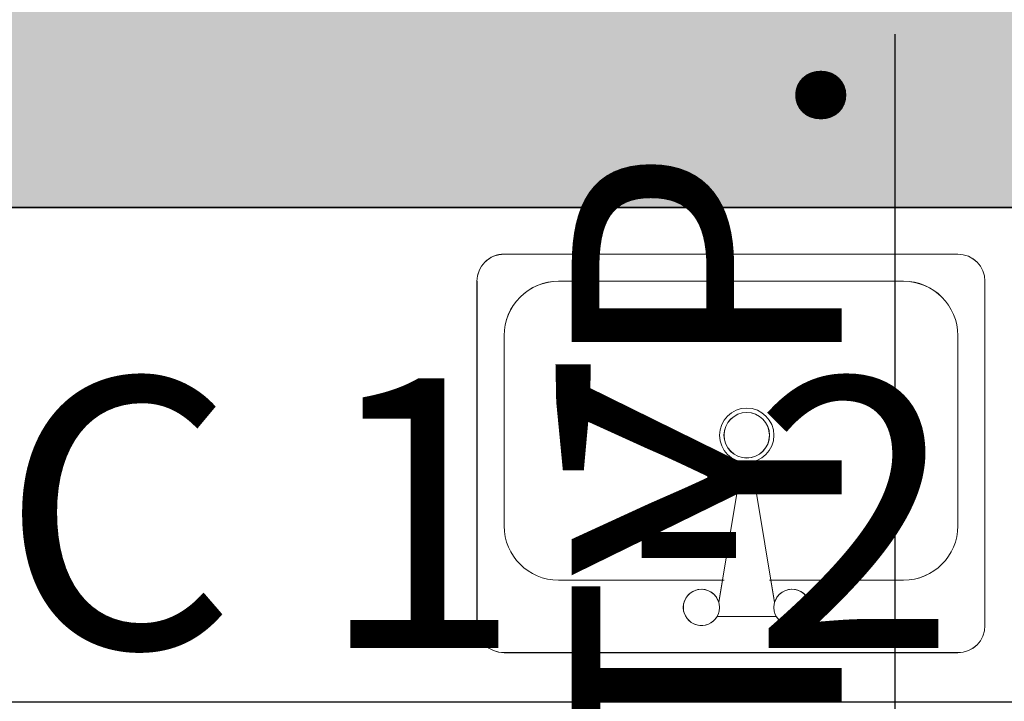
# Model space of a CAD drawing. Units: inches. Extents: x 2083 to 3317, y 1141 to 2115.
# Tile 19 of 256: x 2296 to 2340, y 1447 to 1477. Entities that reach past the tile are written whole.
import ezdxf

# ---------------------------------------------------------------- set-up
doc = ezdxf.new("R2010")
doc.units = ezdxf.units.IN
for name, color, linetype, lineweight in [('A-ANNO-DIMS', 2, 'Continuous', 18), ('A-FLOR-FIXT', 9, 'Continuous', 18), ('A-WALL', 7, 'Continuous', 35)]:
    doc.layers.add(name, color=color, linetype=linetype, lineweight=lineweight)
doc.layers.add('A-WALL-PATT', color=251, linetype='Continuous', lineweight=13, true_color=0x636466)
doc.styles.add('DIM_FONT', font='TXT.shx', dxfattribs={"width": 0.8})
doc.styles.get("Standard").update_dxf_attribs({"font": 'arial.ttf'})
doc.dimstyles.new('ISO-25', dxfattribs={"dimtxt": 12, "dimasz": 12, "dimexe": 1.25, "dimexo": 0.625, "dimtad": 1, "dimlunit": 3, "dimtxsty": 'Standard', "dimcen": 2.5, "dimadec": 0, "dimazin": 0, "dimtfac": 1, "dimtmove": 0, "dimatfit": 3, "dimfxl": 1, "dimarcsym": 0})

# ---------------------------------------------------------------- blocks, each defined once
blk = doc.blocks.new('A$C564A496C')
at = {"linetype": 'ByBlock'}
for p, q in [((543.2, 450), (30.7, 450)), ((0, 419.3), (0, 30.7)), ((573.8, 30.7), (573.8, 419.3)), ((238.5, 409.1), (299.8, 409.1)), ((238.5, 388.6), (258.9, 265.9)), ((279.4, 265.9), (299.8, 388.6)), ((92, 368.2), (243.6, 368.2)), ((294.7, 368.2), (481.8, 368.2)), ((30.7, 92), (30.7, 306.8)), ((543.2, 306.8), (543.2, 92)), ((258.9, 265.9), (279.4, 265.9)), ((481.8, 30.7), (92, 30.7)), ((30.7, 0), (543.2, 0))]:
    blk.add_line(p, q, dxfattribs=at)
for centre, radius in [((218, 398.9), 20.5), ((320.3, 398.9), 20.5), ((269.1, 204.5), 30.7), ((269.1, 204.5), 25.7)]:
    blk.add_circle(centre, radius, dxfattribs=at)
for centre, radius, start, end in [((30.7, 419.3), 30.7, 90, 180), ((543.2, 419.3), 30.7, 0, 90), ((92, 306.8), 61.4, 90, 180), ((481.8, 306.8), 61.4, 0, 90), ((92, 92), 61.4, 180, 270), ((481.8, 92), 61.4, 270, 0), ((30.7, 30.7), 30.7, 180, 270), ((543.2, 30.7), 30.7, 270, 0)]:
    blk.add_arc(centre, radius, start, end, dxfattribs=at)
at = {"style": 'DIM_FONT', "width": 0.8, "flags": 9}
for tag in ['YSIZE', 'XSIZE']:
    blk.add_attdef(tag, (269.1, 450), '', height=0.5, rotation=270, dxfattribs=at)
blk = doc.blocks.new('*D23')
at = {"layer": 'A-ANNO-DIMS', "color": 0, "lineweight": -2, "transparency": 16777216}
for p, q in [((2335.205, 1362.114), (2335.205, 1476.472)), ((2322.885, 1362.114), (2336.455, 1362.114)), ((2335.205, 1306.473), (2335.205, 1350.114)), ((2322.885, 1294.473), (2336.455, 1294.473))]:
    blk.add_line(p, q, dxfattribs=at)
at = {"layer": 'A-ANNO-DIMS', "color": 0, "transparency": 16777216}
for points in [[(2333.205, 1350.114), (2337.205, 1350.114), (2335.205, 1362.114)], [(2333.205, 1306.473), (2337.205, 1306.473), (2335.205, 1294.473)]]:
    blk.add_solid(points, dxfattribs=at)
at = {"layer": 'Defpoints', "color": 0, "transparency": 16777216}
for p in [(2322.26, 1362.114), (2335.205, 1362.114), (2322.26, 1294.473)]:
    blk.add_point(p, dxfattribs=at)
at = {"layer": 'A-ANNO-DIMS', "color": 0, "transparency": 16777216, "insert": (2328.376, 1425.293), "char_height": 12, "attachment_point": 5, "rotation": 90}
blk.add_mtext('5\'-7 1/2" TYP.', dxfattribs=at)
blk = doc.blocks.new('*D30')
at = {"layer": 'A-ANNO-DIMS', "color": 0, "lineweight": -2, "transparency": 16777216}
for p, q in [((2240.018, 1445.274), (2240.018, 1448.046)), ((2254.329, 1445.274), (2254.329, 1448.046)), ((2228.018, 1446.796), (2216.018, 1446.796)), ((2240.018, 1446.796), (2254.329, 1446.796)), ((2266.329, 1446.796), (2413.765, 1446.796))]:
    blk.add_line(p, q, dxfattribs=at)
at = {"layer": 'A-ANNO-DIMS', "color": 0, "transparency": 16777216}
for points in [[(2228.018, 1448.796), (2228.018, 1444.796), (2240.018, 1446.796)], [(2266.329, 1448.796), (2266.329, 1444.796), (2254.329, 1446.796)]]:
    blk.add_solid(points, dxfattribs=at)
at = {"layer": 'Defpoints', "color": 0, "transparency": 16777216}
for p in [(2254.329, 1446.796), (2240.018, 1444.649), (2254.329, 1444.649)]:
    blk.add_point(p, dxfattribs=at)
at = {"layer": 'A-ANNO-DIMS', "color": 0, "transparency": 16777216, "insert": (2346.047, 1453.625), "char_height": 12, "attachment_point": 5}
blk.add_mtext('WC 1\'-2 1/2" TYP.', dxfattribs=at)
blk = doc.blocks.new('*D62')
at = {"layer": 'A-ANNO-DIMS', "color": 0, "lineweight": -2, "transparency": 16777216}
for p, q in [((2235.96, 1469.386), (2235.96, 1522.361)), ((2379.96, 1469.386), (2379.96, 1522.361)), ((2247.96, 1521.111), (2367.96, 1521.111))]:
    blk.add_line(p, q, dxfattribs=at)
at = {"layer": 'A-ANNO-DIMS', "color": 0, "transparency": 16777216}
for points in [[(2247.96, 1523.111), (2247.96, 1519.111), (2235.96, 1521.111)], [(2367.96, 1523.111), (2367.96, 1519.111), (2379.96, 1521.111)]]:
    blk.add_solid(points, dxfattribs=at)
at = {"layer": 'Defpoints', "color": 0, "transparency": 16777216}
for p in [(2379.96, 1521.111), (2235.96, 1468.761), (2379.96, 1468.761)]:
    blk.add_point(p, dxfattribs=at)
at = {"layer": 'A-ANNO-DIMS', "color": 0, "transparency": 16777216, "insert": (2307.96, 1527.863), "char_height": 12, "attachment_point": 5}
blk.add_mtext('12\'-0"', dxfattribs=at)

msp = doc.modelspace()

# ---------------------------------------------------------------- hatches: boundary and pattern name
at = {"layer": 'A-WALL-PATT'}
h = msp.add_hatch(color=256, dxfattribs=at)
h.dxf.hatch_style = 1
h.paths.add_polyline_path([(3126.96, 2020.761), (2748.96, 2020.761), (2604.96, 2020.761), (2226.96, 2020.761), (2226.96, 1702.761), (2466.96, 1702.761), (2466.96, 1582.761), (2418.96, 1582.761), (2418.96, 1477.761), (2226.96, 1477.761), (2226.96, 1263.261), (2544.96, 1263.261), (2544.96, 1411.761), (2604.96, 1411.761), (2685.96, 1411.761), (2685.96, 1420.761), (2604.96, 1420.761), (2604.96, 1573.761), (2604.96, 1702.761), (2604.96, 2011.761), (2748.96, 2011.761), (2748.96, 1702.761), (2862.96, 1702.761), (2862.96, 1621.761), (2871.96, 1621.761), (2871.96, 1702.761), (2883.96, 1702.761), (2883.96, 1706.939, -0.026459), (2883.96, 1711.761), (2757.96, 1711.761), (2757.96, 1807.761), (2787.96, 1807.761), (2787.96, 1812.261), (2757.96, 1812.261), (2757.96, 2011.761), (2877.96, 2011.761), (2877.96, 1812.261), (2847.96, 1812.261), (2847.96, 1807.761), (2889.836, 1807.761), (2889.836, 1812.261), (2882.46, 1812.261), (2882.46, 2011.761), (3117.96, 2011.761), (3117.96, 1812.261), (2937.836, 1812.261), (2937.836, 1807.761), (2995.71, 1807.761), (2995.71, 1796.118), (3000.21, 1796.118), (3000.21, 1807.761), (3117.96, 1807.761), (3117.96, 1711.761), (3000.21, 1711.761), (3000.21, 1760.118), (2998.573, 1760.118, -0.020711), (2995.71, 1760.118), (2995.71, 1711.761), (2931.96, 1711.761), (2931.96, 1702.761), (3126.96, 1702.761)])
h.paths.add_polyline_path([(2471.46, 2011.761), (2471.46, 1810.011), (2462.717, 1810.011), (2462.717, 1805.511), (2505.96, 1805.511), (2505.96, 1810.011), (2475.96, 1810.011), (2475.96, 2011.761), (2595.96, 2011.761), (2595.96, 1810.011), (2565.96, 1810.011), (2565.96, 1805.511), (2595.96, 1805.511), (2595.96, 1711.761), (2235.96, 1711.761), (2235.96, 1805.511), (2353.71, 1805.511), (2353.71, 1796.054), (2358.21, 1796.054), (2358.21, 1805.511), (2414.717, 1805.511), (2414.717, 1810.011), (2235.96, 1810.011), (2235.96, 2011.761)], flags=16)
h.paths.add_polyline_path([(2270.205, 1994.61), (2270.205, 1970.61), (2246.205, 1970.61), (2246.205, 1994.61)], flags=0)
edge = h.paths.add_edge_path(flags=0)
edge.add_ellipse((2332.027, 1899.798), major_axis=(-3.043, 3.043), ratio=0.168252, start_angle=-161.3322, end_angle=-156.3071, ccw=False)
edge.add_ellipse((2333.082, 1898.744), major_axis=(-1.055, 1.055), ratio=0.453532, start_angle=-123.371, end_angle=-94.1591)
edge = h.paths.add_edge_path(flags=0)
edge.add_ellipse((2332.027, 1968.876), major_axis=(3.043, 3.043), ratio=0.168252, start_angle=18.6678, end_angle=23.6929)
edge.add_spline(control_points=[(2332.926, 1970.691), (2332.227, 1970.336), (2330.894, 1969.659), (2328.413, 1970.932), (2327.204, 1967.749), (2324.71, 1969.956), (2322.533, 1967.012), (2320.013, 1971.296), (2317.68, 1968.158), (2316.041, 1967.102), (2315.427, 1966.81)], knot_values=[0, 0, 0, 0, 2.267059, 4.324559, 6.685584, 8.878641, 11.121502, 14.300359, 17.755284, 19.732645, 19.732645, 19.732645, 19.732645], degree=3, periodic=0)
edge.add_ellipse((2332.027, 1968.876), major_axis=(3.043, 3.043), ratio=0.168252, start_angle=18.6678, end_angle=23.6929, ccw=False)
edge.add_ellipse((2333.082, 1969.931), major_axis=(1.055, 1.055), ratio=0.453532, start_angle=56.629, end_angle=85.8409, ccw=False)
edge = h.paths.add_edge_path(flags=0)
edge.add_spline(control_points=[(2296.428, 1967.988), (2293.628, 1965.336), (2287.704, 1959.727), (2299.744, 1949.996), (2294.533, 1935.669), (2290.573, 1920.604), (2293.394, 1909.974), (2296.185, 1904.967)], knot_values=[0.099185, 0.099185, 0.099185, 0.099185, 0.345301, 0.619822, 0.982653, 1.386093, 1.810555, 1.810555, 1.810555, 1.810555], degree=3, periodic=0)
edge.add_spline(control_points=[(2296.185, 1904.967), (2297.384, 1902.619), (2298.001, 1901.949), (2298.553, 1901.468)], knot_values=[0.006246, 0.006246, 0.006246, 0.006246, 0.055476, 0.055476, 0.055476, 0.055476], degree=3, periodic=0)
edge.add_spline(control_points=[(2298.553, 1901.468), (2297.259, 1900.923), (2295.225, 1900.232), (2293.06, 1900.614), (2292.101, 1900.788), (2292.09, 1900.791)], knot_values=[0.312835, 0.312835, 0.312835, 0.312835, 0.40178, 0.474987, 0.475903, 0.475903, 0.475903, 0.475903], degree=3, periodic=0)
edge.add_arc((2292.794, 1904.664), 3.937, 215.4209, 259.6982, ccw=False)
edge.add_spline(control_points=[(2289.585, 1902.382), (2289.477, 1902.535), (2289.368, 1902.688), (2289.261, 1902.841)], knot_values=[0.102872, 0.102872, 0.102872, 0.102872, 0.116896, 0.116896, 0.116896, 0.116896], degree=3, periodic=0)
edge.add_spline(control_points=[(2289.261, 1902.841), (2288.687, 1902.55), (2287.64, 1902.02), (2285.881, 1901.874), (2283.853, 1901.504), (2281.72, 1899.711), (2278.467, 1899.493), (2276.157, 1901.883), (2272.259, 1899.804), (2267.778, 1901.843), (2262.244, 1900.184), (2257.415, 1901.782), (2254.318, 1900.726), (2253.178, 1900.337)], knot_values=[0, 0, 0, 0, 1.907977, 3.477176, 5.261074, 7.972851, 11.680248, 13.717921, 16.939592, 22.789562, 27.502503, 33.595215, 37.145618, 37.145618, 37.145618, 37.145618], degree=3, periodic=0)
edge.add_line((2253.178, 1900.337), (2250.244, 1902.841))
edge.add_line((2250.244, 1902.841), (2250.244, 1965.833))
edge.add_line((2250.244, 1965.833), (2253.178, 1968.337))
edge.add_spline(control_points=[(2253.178, 1968.337), (2254.318, 1967.948), (2257.415, 1966.892), (2262.244, 1968.49), (2267.778, 1966.831), (2271.527, 1968.537), (2273.876, 1967.828), (2274.207, 1967.728)], knot_values=[0, 0, 0, 0, 0.09018, 0.244935, 0.364644, 0.513233, 0.537855, 0.537855, 0.537855, 0.537855], degree=3, periodic=0)
edge.add_arc((2274.353, 1963.793), 3.937, 72.0511, 92.1279, ccw=False)
edge.add_arc((2281.297, 1985.23), 18.596, 252.0511, 288.5657)
edge.add_arc((2292.317, 1956.029), 12.646, 71.0268, 113.7782, ccw=False)
edge = h.paths.add_edge_path(flags=0)
edge.add_spline(control_points=[(2274.899, 1951.856), (2275.066, 1951.617), (2275.233, 1951.377), (2275.398, 1951.136)], knot_values=[1.409916, 1.409916, 1.409916, 1.409916, 1.43159, 1.43159, 1.43159, 1.43159], degree=3, periodic=0)
edge.add_spline(control_points=[(2275.398, 1951.136), (2275.792, 1950.562), (2276.179, 1949.984), (2276.546, 1949.397)], knot_values=[1.358238, 1.358238, 1.358238, 1.358238, 1.409916, 1.409916, 1.409916, 1.409916], degree=3, periodic=0)
edge.add_line((2276.546, 1949.397), (2277.437, 1947.862))
edge.add_spline(control_points=[(2277.437, 1947.862), (2276.304, 1945.673), (2274.64, 1942.427), (2274.632, 1938.094), (2272.799, 1930.852), (2274.356, 1943.897), (2275.948, 1947.923), (2276.546, 1949.397)], knot_values=[0.005632, 0.005632, 0.005632, 0.005632, 0.186014, 0.266002, 0.357087, 0.59639, 0.739732, 0.739732, 0.739732, 0.739732], degree=3, periodic=0)
edge.add_spline(control_points=[(2276.546, 1949.397), (2276.179, 1949.984), (2275.792, 1950.562), (2275.398, 1951.136)], knot_values=[1.358238, 1.358238, 1.358238, 1.358238, 1.409916, 1.409916, 1.409916, 1.409916], degree=3, periodic=0)
edge.add_spline(control_points=[(2275.398, 1951.136), (2274.943, 1950.08), (2274.208, 1948.025), (2273.935, 1944.851), (2272.469, 1937.627), (2273.466, 1945.696), (2274.701, 1951.059), (2274.899, 1951.856)], knot_values=[0.104364, 0.104364, 0.104364, 0.104364, 0.189636, 0.269624, 0.36071, 0.600013, 0.644622, 0.644622, 0.644622, 0.644622], degree=3, periodic=0)
h.paths.add_polyline_path([(2269.168, 1963.128, -0.357527), (2268.171, 1960.976, -0.092561), (2268.171, 1939.436, -0.357527), (2269.168, 1937.285, -0.357527), (2267.016, 1938.282, -0.164785), (2254.686, 1938.282, -0.357527), (2252.534, 1937.285, -0.357527), (2253.531, 1939.436, -0.092561), (2253.531, 1960.976, -0.357527), (2252.534, 1963.128, -0.357527), (2254.686, 1962.131, -0.164785), (2267.016, 1962.131, -0.357527)], flags=0)
h.paths.add_polyline_path([(2248.874, 1967.802), (2248.874, 1957.028), (2249.458, 1957.028), (2249.458, 1911.647), (2248.874, 1911.647), (2248.874, 1900.873), (2246.512, 1900.873, 0.197327), (2244.15, 1902.457), (2244.15, 1966.218, 0.197327), (2246.512, 1967.802)], flags=0)
h.paths.add_polyline_path([(2269.168, 1931.389, -0.357527), (2268.171, 1929.238, -0.092561), (2268.171, 1907.698, -0.357527), (2269.168, 1905.547, -0.357527), (2267.016, 1906.544, -0.164785), (2254.686, 1906.544, -0.357527), (2252.534, 1905.547, -0.357527), (2253.531, 1907.698, -0.092561), (2253.531, 1929.238, -0.357527), (2252.534, 1931.389, -0.357527), (2254.686, 1930.392, -0.164785), (2267.016, 1930.392, -0.357527)], flags=0)
edge = h.paths.add_edge_path(flags=0)
edge.add_spline(control_points=[(2276.197, 1906.724), (2276.168, 1909.029), (2276.114, 1913.372), (2270.598, 1924.925), (2273.905, 1919.013), (2275.922, 1916.262), (2275.475, 1912.402), (2277.258, 1910.381), (2276.696, 1908.225), (2276.646, 1906.813), (2276.618, 1906.008)], knot_values=[0, 0, 0, 0, 8.61026, 16.221274, 18.843057, 23.804898, 27.440828, 29.356102, 31.203478, 33.650687, 33.650687, 33.650687, 33.650687], degree=3, periodic=0)
edge.add_spline(control_points=[(2276.618, 1906.008), (2276.623, 1905.624), (2276.498, 1904.629), (2275.442, 1903.855), (2274.937, 1903.08), (2274.859, 1902.841)], knot_values=[0.156488, 0.156488, 0.156488, 0.156488, 0.184398, 0.231376, 0.250598, 0.250598, 0.250598, 0.250598], degree=3, periodic=0)
edge.add_line((2274.859, 1902.841), (2276.506, 1902.841))
edge.add_spline(control_points=[(2276.506, 1902.841), (2276.788, 1903.085), (2277.665, 1904.125), (2278.25, 1904.341), (2277.654, 1908.527), (2278.156, 1906.228), (2278.1, 1905.286), (2278.847, 1904.069), (2277.857, 1903.415), (2277.874, 1902.991), (2277.904, 1902.841)], knot_values=[0.059574, 0.059574, 0.059574, 0.059574, 0.080753, 0.103741, 0.16972, 0.176036, 0.207137, 0.240474, 0.262341, 0.27366, 0.27366, 0.27366, 0.27366], degree=3, periodic=0)
edge.add_line((2277.904, 1902.841), (2280.03, 1902.841))
edge.add_spline(control_points=[(2280.03, 1902.841), (2279.888, 1903.088), (2279.499, 1903.982), (2280.152, 1905.939), (2278.104, 1909.658), (2279.762, 1907.185), (2280.328, 1904.875), (2280.485, 1903.49), (2281.463, 1903.249), (2281.758, 1902.936), (2281.834, 1902.841)], knot_values=[0.013856, 0.013856, 0.013856, 0.013856, 0.034874, 0.088867, 0.107879, 0.126738, 0.158714, 0.193757, 0.217487, 0.226722, 0.226722, 0.226722, 0.226722], degree=3, periodic=0)
edge.add_spline(control_points=[(2281.834, 1902.841), (2281.788, 1902.827), (2281.647, 1902.783), (2281.396, 1902.859), (2281.088, 1902.985), (2280.721, 1903.061), (2280.333, 1903.026), (2280.125, 1902.899), (2280.03, 1902.841)], knot_values=[0, 0, 0, 0, 0.14413, 0.435517, 0.749276, 1.153046, 1.548371, 1.878348, 1.878348, 1.878348, 1.878348], degree=3, periodic=0)
edge.add_line((2280.03, 1902.841), (2277.904, 1902.841))
edge.add_spline(control_points=[(2277.904, 1902.841), (2277.893, 1902.796), (2277.865, 1902.68), (2277.607, 1902.687), (2277.274, 1902.801), (2276.838, 1902.62), (2276.584, 1902.789), (2276.506, 1902.841)], knot_values=[0, 0, 0, 0, 0.127189, 0.326199, 0.628009, 1.24357, 1.515331, 1.515331, 1.515331, 1.515331], degree=3, periodic=0)
edge.add_line((2276.506, 1902.841), (2274.859, 1902.841))
edge.add_spline(control_points=[(2274.859, 1902.841), (2274.814, 1902.899), (2274.725, 1903.013), (2274.493, 1903.119), (2274.244, 1902.961), (2273.937, 1903.185), (2273.614, 1902.983), (2273.408, 1902.883), (2273.322, 1902.841)], knot_values=[0, 0, 0, 0, 0.21843, 0.436957, 0.687977, 0.990379, 1.398396, 1.69185, 1.69185, 1.69185, 1.69185], degree=3, periodic=0)
edge.add_spline(control_points=[(2273.322, 1902.841), (2273.617, 1903.446), (2274.274, 1904.538), (2276.027, 1904.574), (2276.207, 1906.584), (2276.197, 1906.724)], knot_values=[0.012227, 0.012227, 0.012227, 0.012227, 0.059472, 0.106218, 0.134458, 0.134458, 0.134458, 0.134458], degree=3, periodic=0)
h.paths.add_polyline_path([(2270.776, 1897.79), (2270.776, 1873.79), (2246.776, 1873.79), (2246.776, 1897.79)], flags=0)
h.paths.add_polyline_path([(2353.71, 1760.005), (2353.71, 1760.054), (2358.21, 1760.054, -0.033729)], flags=0)
h.paths.add_polyline_path([(2321.819, 1737.529), (2341.995, 1737.529, -0.414214), (2343.203, 1736.321), (2343.203, 1721.021, -0.414214), (2341.995, 1719.813), (2321.819, 1719.813, -0.414214), (2320.611, 1721.021), (2320.611, 1736.321, -0.414214)], flags=0)
h.paths.add_polyline_path([(2324.235, 1736.321), (2339.579, 1736.321, -0.414214), (2341.995, 1733.905), (2341.995, 1725.45, -0.414214), (2339.579, 1723.034), (2333.681, 1723.034), (2333.845, 1722.045, -0.870646), (2335.425, 1721.826, -0.767327), (2333.923, 1721.423), (2331.291, 1721.423, -0.767327), (2329.788, 1721.826, -0.870646), (2331.368, 1722.045), (2331.533, 1723.034), (2324.235, 1723.034, -0.414214), (2321.819, 1725.45), (2321.819, 1733.905, -0.414214)], flags=0)
h.paths.add_polyline_path([(2570.484, 1928.615), (2589.684, 1928.615), (2590.169, 1928.615), (2590.169, 1904.993), (2570.484, 1904.993)], flags=0)
h.paths.add_polyline_path([(2574.447, 1927.264, -1), (2572.829, 1927.264, -1)], flags=0)
h.paths.add_polyline_path([(2573.09, 1926.941), (2573.925, 1927.776), (2574.148, 1927.553), (2573.313, 1926.718)], flags=0)
h.paths.add_polyline_path([(2578.779, 1919.73, -1), (2571.592, 1919.73, -1)], flags=0)
h.paths.add_polyline_path([(2578.385, 1919.73, -1), (2571.985, 1919.73, -1)], flags=0)
h.paths.add_polyline_path([(2331.596, 1729.476, -1), (2333.618, 1729.476, -1)], flags=0)
h.paths.add_polyline_path([(2578.034, 1927.264, -1), (2576.416, 1927.264, -1)], flags=0)
h.paths.add_polyline_path([(2576.689, 1927.531), (2576.912, 1927.754), (2577.747, 1926.919), (2577.524, 1926.696)], flags=0)
h.paths.add_polyline_path([(2578.139, 1909.86, -1), (2572.232, 1909.86, -1)], flags=0)
h.paths.add_polyline_path([(2577.745, 1909.86, -1), (2572.625, 1909.86, -1)], flags=0)
h.paths.add_polyline_path([(2583.798, 1927.264, -1), (2582.179, 1927.264, -1)], flags=0)
h.paths.add_polyline_path([(2582.719, 1927.754), (2583.554, 1926.919), (2583.331, 1926.696), (2582.496, 1927.531)], flags=0)
h.paths.add_polyline_path([(2582.496, 1927.531), (2582.719, 1927.754), (2583.554, 1926.919), (2583.331, 1926.696)], flags=0)
h.paths.add_polyline_path([(2587.739, 1920.53, -1), (2581.832, 1920.53, -1)], flags=0)
h.paths.add_polyline_path([(2587.345, 1920.53, -1), (2582.225, 1920.53, -1)], flags=0)
h.paths.add_polyline_path([(2587.385, 1927.264, -1), (2585.766, 1927.264, -1)], flags=0)
h.paths.add_polyline_path([(2586.082, 1926.98), (2586.917, 1927.815), (2587.14, 1927.593), (2586.305, 1926.758)], flags=0)
h.paths.add_polyline_path([(2588.379, 1910.66, -1), (2581.192, 1910.66, -1)], flags=0)
h.paths.add_polyline_path([(2587.985, 1910.66, -1), (2581.585, 1910.66, -1)], flags=0)
h.paths.add_polyline_path([(2417.168, 1729.478), (2437.344, 1729.478, -0.414214), (2438.552, 1728.27), (2438.552, 1712.969, -0.414214), (2437.344, 1711.761), (2417.168, 1711.761, -0.414214), (2415.96, 1712.969), (2415.96, 1728.27, -0.414214)], flags=0)
h.paths.add_polyline_path([(2419.584, 1728.27), (2434.928, 1728.27, -0.414214), (2437.344, 1725.854), (2437.344, 1717.398, -0.414214), (2434.928, 1714.983), (2429.029, 1714.983), (2429.194, 1713.994, -0.870646), (2430.774, 1713.775, -0.767327), (2429.271, 1713.372), (2426.64, 1713.372, -0.767327), (2425.137, 1713.775, -0.870646), (2426.717, 1713.994), (2426.882, 1714.983), (2419.584, 1714.983, -0.414214), (2417.168, 1717.398), (2417.168, 1725.854, -0.414214)], flags=0)
h.paths.add_polyline_path([(2419.584, 1728.27), (2434.928, 1728.27, -0.414214), (2437.344, 1725.854), (2437.344, 1717.398, -0.414214), (2434.928, 1714.983), (2429.029, 1714.983), (2428.358, 1719.009), (2427.553, 1719.009), (2426.882, 1714.983), (2419.584, 1714.983, -0.414214), (2417.168, 1717.398), (2417.168, 1725.854, -0.414214)], flags=0)
h.paths.add_polyline_path([(2426.944, 1721.425, -1), (2428.967, 1721.425, -1)], flags=0)
h.paths.add_polyline_path([(2475.96, 1702.761), (2595.96, 1702.761), (2595.96, 1582.761), (2475.96, 1582.761)], flags=16)
h.paths.add_polyline_path([(2427.96, 1573.761), (2595.96, 1573.761), (2595.96, 1468.761), (2595.96, 1420.761), (2384.46, 1420.761), (2384.46, 1468.761), (2427.96, 1468.761)], flags=16)
h.paths.add_polyline_path([(2379.96, 1468.761), (2379.96, 1420.761), (2235.96, 1420.761), (2235.96, 1468.761)], flags=16)
h.paths.add_polyline_path([(2317.816, 1466.696), (2337.992, 1466.696, -0.414214), (2339.2, 1465.488), (2339.2, 1450.187, -0.414214), (2337.992, 1448.979), (2317.816, 1448.979, -0.414214), (2316.608, 1450.187), (2316.608, 1465.488, -0.414214)], flags=0)
h.paths.add_polyline_path([(2320.232, 1465.488), (2335.576, 1465.488, -0.414214), (2337.992, 1463.072), (2337.992, 1454.616, -0.414214), (2335.576, 1452.2), (2329.677, 1452.2), (2329.842, 1451.212, -0.870646), (2331.422, 1450.992, -0.767327), (2329.92, 1450.59), (2327.288, 1450.59, -0.767327), (2325.785, 1450.992, -0.870646), (2327.365, 1451.212), (2327.53, 1452.2), (2320.232, 1452.2, -0.414214), (2317.816, 1454.616), (2317.816, 1463.072, -0.414214)], flags=0)
h.paths.add_polyline_path([(2320.232, 1465.488), (2335.576, 1465.488, -0.414214), (2337.992, 1463.072), (2337.992, 1454.616, -0.414214), (2335.576, 1452.2), (2329.677, 1452.2), (2329.006, 1456.227), (2328.201, 1456.227), (2327.53, 1452.2), (2320.232, 1452.2, -0.414214), (2317.816, 1454.616), (2317.816, 1463.072, -0.414214)], flags=0)
h.paths.add_polyline_path([(2327.593, 1458.643, -1), (2329.615, 1458.643, -1)], flags=0)
h.paths.add_polyline_path([(2244.412, 1433.34), (2241.921, 1433.34, -0.414214), (2240.018, 1435.244), (2240.018, 1440.953, -0.414211), (2241.921, 1442.856), (2244.412, 1442.856, -1.976472)], flags=0)
h.paths.add_polyline_path([(2245.357, 1434.398, -0.414214), (2245.357, 1441.799, -2.144098)], flags=0)
h.paths.add_polyline_path([(2535.96, 1416.261), (2535.96, 1272.261), (2235.96, 1272.261), (2235.96, 1416.261)], flags=16)
h.paths.add_polyline_path([(2260.12, 1384.293), (2260.12, 1362.039), (2237.865, 1362.039), (2237.865, 1384.293)], flags=0)
edge = h.paths.add_edge_path(flags=0)
edge.add_line((2318.252, 1362.093), (2318.146, 1362.001))
edge.add_ellipse((2317.445, 1360.431), major_axis=(2.822, 2.822), ratio=0.168252, start_angle=18.6678, end_angle=20.9481, ccw=False)
edge.add_ellipse((2318.423, 1361.409), major_axis=(0.978, 0.978), ratio=0.453532, start_angle=56.629, end_angle=70.2262, ccw=False)
edge = h.paths.add_edge_path(flags=0)
edge.add_line((2319.107, 1295.571), (2319.015, 1295.677))
edge.add_ellipse((2317.445, 1296.378), major_axis=(-2.822, 2.822), ratio=0.168252, start_angle=-161.3322, end_angle=-159.0519, ccw=False)
edge.add_ellipse((2318.423, 1295.4), major_axis=(-0.978, 0.978), ratio=0.453532, start_angle=-123.371, end_angle=-109.7738)
edge = h.paths.add_edge_path(flags=0)
edge.add_spline(control_points=[(2284.21, 1301.17), (2284.581, 1300.445), (2284.891, 1299.892), (2285.16, 1299.461)], knot_values=[0.039066, 0.039066, 0.039066, 0.039066, 0.055476, 0.055476, 0.055476, 0.055476], degree=3, periodic=0)
edge.add_line((2285.16, 1299.461), (2284.21, 1301.17))
edge = h.paths.add_edge_path(flags=0)
edge.add_line((2280.412, 1297.298), (2283.37, 1297.036))
edge.add_line((2283.37, 1297.036), (2286.406, 1297.926))
edge.add_spline(control_points=[(2286.406, 1297.926), (2285.305, 1297.463), (2284.345, 1297.129), (2283.37, 1297.036)], knot_values=[0.394369, 0.394369, 0.394369, 0.394369, 0.475903, 0.475903, 0.475903, 0.475903], degree=3, periodic=0)
edge.add_spline(control_points=[(2283.37, 1297.036), (2283.281, 1297.028), (2282.316, 1296.957), (2281.313, 1297.134), (2280.423, 1297.296), (2280.412, 1297.298)], knot_values=[0.312835, 0.312835, 0.312835, 0.312835, 0.320246, 0.393453, 0.394369, 0.394369, 0.394369, 0.394369], degree=3, periodic=0)
edge = h.paths.add_edge_path(flags=0)
edge.add_line((2284.436, 1359.607), (2280.446, 1355.328))
edge.add_line((2280.446, 1355.328), (2279.58, 1351.018))
edge.add_line((2279.58, 1351.018), (2282.413, 1346.58))
edge.add_spline(control_points=[(2282.413, 1346.58), (2283.153, 1345.589), (2284.253, 1344.029), (2284.801, 1342.387), (2284.935, 1341.806)], knot_values=[1.240098, 1.240098, 1.240098, 1.240098, 1.332892, 1.382712, 1.382712, 1.382712, 1.382712], degree=3, periodic=0)
edge.add_spline(control_points=[(2284.935, 1341.806), (2285.319, 1340.141), (2285.233, 1338.409), (2284.91, 1336.654)], knot_values=[1.097484, 1.097484, 1.097484, 1.097484, 1.240098, 1.240098, 1.240098, 1.240098], degree=3, periodic=0)
edge.add_spline(control_points=[(2284.91, 1336.654), (2284.587, 1334.899), (2284.027, 1333.12), (2283.463, 1331.361)], knot_values=[0.95487, 0.95487, 0.95487, 0.95487, 1.097484, 1.097484, 1.097484, 1.097484], degree=3, periodic=0)
edge.add_line((2283.463, 1331.361), (2281.89, 1326.153))
edge.add_line((2281.89, 1326.153), (2280.756, 1321.056))
edge.add_line((2280.756, 1321.056), (2280.299, 1316.002))
edge.add_line((2280.299, 1316.002), (2280.716, 1310.95))
edge.add_line((2280.716, 1310.95), (2282.028, 1305.972))
edge.add_line((2282.028, 1305.972), (2284.21, 1301.17))
edge.add_spline(control_points=[(2284.21, 1301.17), (2283.341, 1302.73), (2282.612, 1304.336), (2282.028, 1305.972)], knot_values=[0.099185, 0.099185, 0.099185, 0.099185, 0.241799, 0.241799, 0.241799, 0.241799], degree=3, periodic=0)
edge.add_spline(control_points=[(2282.028, 1305.972), (2281.444, 1307.608), (2281.005, 1309.273), (2280.716, 1310.95)], knot_values=[0.241799, 0.241799, 0.241799, 0.241799, 0.384413, 0.384413, 0.384413, 0.384413], degree=3, periodic=0)
edge.add_spline(control_points=[(2280.716, 1310.95), (2280.433, 1312.588), (2280.289, 1314.277), (2280.299, 1315.962), (2280.299, 1316.002)], knot_values=[0.384413, 0.384413, 0.384413, 0.384413, 0.523647, 0.527028, 0.527028, 0.527028, 0.527028], degree=3, periodic=0)
edge.add_spline(control_points=[(2280.299, 1316.002), (2280.312, 1317.687), (2280.478, 1319.368), (2280.756, 1321.056)], knot_values=[0.527028, 0.527028, 0.527028, 0.527028, 0.669642, 0.669642, 0.669642, 0.669642], degree=3, periodic=0)
edge.add_spline(control_points=[(2280.756, 1321.056), (2281.035, 1322.744), (2281.426, 1324.44), (2281.89, 1326.153)], knot_values=[0.669642, 0.669642, 0.669642, 0.669642, 0.812256, 0.812256, 0.812256, 0.812256], degree=3, periodic=0)
edge.add_spline(control_points=[(2281.89, 1326.153), (2282.264, 1327.533), (2282.788, 1329.262), (2283.353, 1331.018), (2283.463, 1331.361)], knot_values=[0.812256, 0.812256, 0.812256, 0.812256, 0.927087, 0.95487, 0.95487, 0.95487, 0.95487], degree=3, periodic=0)
edge.add_line((2283.463, 1331.361), (2284.91, 1336.654))
edge.add_line((2284.91, 1336.654), (2284.935, 1341.806))
edge.add_line((2284.935, 1341.806), (2282.413, 1346.58))
edge.add_spline(control_points=[(2282.413, 1346.58), (2281.275, 1348.104), (2280.078, 1349.57), (2279.58, 1351.018)], knot_values=[1.382712, 1.382712, 1.382712, 1.382712, 1.525326, 1.525326, 1.525326, 1.525326], degree=3, periodic=0)
edge.add_spline(control_points=[(2279.58, 1351.018), (2279.443, 1351.415), (2279.136, 1352.857), (2279.735, 1354.29), (2280.446, 1355.328)], knot_values=[1.525326, 1.525326, 1.525326, 1.525326, 1.564439, 1.667941, 1.667941, 1.667941, 1.667941], degree=3, periodic=0)
edge.add_spline(control_points=[(2280.446, 1355.328), (2281.426, 1356.758), (2282.931, 1358.183), (2284.436, 1359.607)], knot_values=[1.667941, 1.667941, 1.667941, 1.667941, 1.810555, 1.810555, 1.810555, 1.810555], degree=3, periodic=0)
edge.add_arc((2280.623, 1348.518), 11.726, 71.0268, 113.7782)
edge.add_arc((2270.405, 1375.595), 17.244, 252.0511, 288.5657, ccw=False)
edge.add_arc((2263.966, 1355.718), 3.651, 72.0511, 92.1279)
edge.add_arc((2263.966, 1355.718), 3.651, 92.1279, 177.9851)
edge.add_spline(control_points=[(2260.318, 1355.846), (2260.26, 1354.221), (2260.551, 1350.187), (2262.999, 1346.766), (2264.473, 1344.649)], knot_values=[1.43159, 1.43159, 1.43159, 1.43159, 1.564144, 1.770695, 1.770695, 1.770695, 1.770695], degree=3, periodic=0)
edge.add_line((2264.473, 1344.649), (2264.936, 1343.983))
edge.add_spline(control_points=[(2263.801, 1340.248), (2263.843, 1340.514), (2264.067, 1341.756), (2264.513, 1343.002), (2264.935, 1343.981)], knot_values=[0.53657, 0.53657, 0.53657, 0.53657, 0.559349, 0.644622, 0.644622, 0.644622, 0.644622], degree=3, periodic=0)
edge.add_spline(control_points=[(2264.935, 1343.981), (2265.118, 1343.715), (2265.299, 1343.448), (2265.477, 1343.179)], knot_values=[1.384077, 1.384077, 1.384077, 1.384077, 1.409916, 1.409916, 1.409916, 1.409916], degree=3, periodic=0)
edge.add_spline(control_points=[(2265.477, 1343.179), (2265.655, 1342.911), (2265.829, 1342.641), (2265.999, 1342.369)], knot_values=[1.358238, 1.358238, 1.358238, 1.358238, 1.384077, 1.384077, 1.384077, 1.384077], degree=3, periodic=0)
edge.add_line((2265.999, 1342.369), (2266.826, 1340.946))
edge.add_spline(control_points=[(2266.826, 1340.946), (2268.894, 1337.09), (2271.398, 1325.843), (2270.516, 1310.569), (2275.919, 1301.861), (2277.79, 1299.199)], knot_values=[0.116896, 0.116896, 0.116896, 0.116896, 0.472987, 1.050969, 1.313793, 1.313793, 1.313793, 1.313793], degree=3, periodic=0)
edge.add_spline(control_points=[(2277.79, 1299.199), (2277.839, 1299.128), (2277.889, 1299.057), (2277.94, 1298.987)], knot_values=[0.109884, 0.109884, 0.109884, 0.109884, 0.116896, 0.116896, 0.116896, 0.116896], degree=3, periodic=0)
edge.add_line((2277.94, 1298.987), (2277.789, 1299.199))
edge.add_spline(control_points=[(2277.789, 1299.199), (2277.257, 1298.929), (2276.286, 1298.438), (2275.039, 1298.334), (2274.383, 1298.239), (2274.215, 1298.209)], knot_values=[33.12187, 33.12187, 33.12187, 33.12187, 35.029056, 36.598255, 37.144827, 37.144827, 37.144827, 37.144827], degree=3, periodic=0)
edge.add_line((2274.215, 1298.209), (2273.073, 1297.893))
edge.add_spline(control_points=[(2273.073, 1297.893), (2272.323, 1297.58), (2271.039, 1296.511), (2269.248, 1296.226), (2268.423, 1296.375)], knot_values=[26.532584, 26.532584, 26.532584, 26.532584, 29.198919, 31.839101, 31.839101, 31.839101, 31.839101], degree=3, periodic=0)
edge.add_line((2268.423, 1296.375), (2263.879, 1297.458))
edge.add_spline(control_points=[(2263.879, 1297.458), (2263.556, 1297.359), (2261.86, 1296.839), (2260.239, 1297.282), (2258.933, 1297.516)], knot_values=[15.919551, 15.919551, 15.919551, 15.919551, 16.939592, 21.226067, 21.226067, 21.226067, 21.226067], degree=3, periodic=0)
edge.add_line((2258.933, 1297.516), (2254.055, 1297.329))
edge.add_spline(control_points=[(2254.055, 1297.329), (2253.756, 1297.296), (2252.114, 1297.165), (2250.462, 1297.544), (2249.13, 1297.668)], knot_values=[5.306517, 5.306517, 5.306517, 5.306517, 6.276435, 10.613034, 10.613034, 10.613034, 10.613034], degree=3, periodic=0)
edge.add_line((2249.13, 1297.668), (2244.332, 1296.878))
edge.add_line((2244.332, 1296.878), (2241.611, 1299.199))
edge.add_line((2241.611, 1299.199), (2241.611, 1357.609))
edge.add_line((2241.611, 1357.609), (2244.332, 1359.931))
edge.add_line((2244.332, 1359.931), (2252.729, 1359.543))
edge.add_spline(control_points=[(2252.729, 1359.543), (2252.871, 1359.546), (2253.306, 1359.548), (2253.74, 1359.514), (2254.032, 1359.482)], knot_values=[0.233291, 0.233291, 0.233291, 0.233291, 0.244935, 0.268927, 0.268927, 0.268927, 0.268927], degree=3, periodic=0)
edge.add_line((2254.032, 1359.482), (2259.587, 1359.416))
edge.add_spline(control_points=[(2259.587, 1359.416), (2260.677, 1359.629), (2262.073, 1359.897), (2263.524, 1359.459), (2263.83, 1359.366)], knot_values=[0.422516, 0.422516, 0.422516, 0.422516, 0.513233, 0.537855, 0.537855, 0.537855, 0.537855], degree=3, periodic=0)
edge.add_arc((2263.966, 1355.718), 3.651, 72.0511, 92.1279, ccw=False)
edge.add_arc((2270.405, 1375.595), 17.244, 252.0511, 288.5657)
edge.add_arc((2280.623, 1348.518), 11.726, 71.0268, 113.7782, ccw=False)
h.paths.add_polyline_path([(2240.341, 1359.435), (2240.341, 1349.444), (2240.882, 1349.444), (2240.882, 1307.365), (2240.341, 1307.365), (2240.341, 1297.374), (2238.15, 1297.374, 0.197327), (2235.96, 1298.843), (2235.96, 1357.966, 0.197327), (2238.15, 1359.435)], flags=0)
h.paths.add_polyline_path([(2259.158, 1355.101, -0.357527), (2258.233, 1353.106, -0.092561), (2258.233, 1333.133, -0.357527), (2259.158, 1331.138, -0.357527), (2257.163, 1332.062, -0.164785), (2245.729, 1332.062, -0.357527), (2243.735, 1331.138, -0.357527), (2244.659, 1333.133, -0.092561), (2244.659, 1353.106, -0.357527), (2243.735, 1355.101, -0.357527), (2245.729, 1354.176, -0.164785), (2257.163, 1354.176, -0.357527)], flags=0)
edge = h.paths.add_edge_path(flags=0)
edge.add_line((2265.999, 1342.369), (2266.826, 1340.946))
edge.add_line((2266.826, 1340.946), (2265.308, 1337.814))
edge.add_line((2265.308, 1337.814), (2264.358, 1334.653))
edge.add_line((2264.358, 1334.653), (2264.262, 1333.8))
edge.add_spline(control_points=[(2264.262, 1333.8), (2264.208, 1333.187), (2264.162, 1332.366), (2264.007, 1331.414), (2263.969, 1331.202)], knot_values=[0.464444, 0.464444, 0.464444, 0.464444, 0.516691, 0.531608, 0.531608, 0.531608, 0.531608], degree=3, periodic=0)
edge.add_spline(control_points=[(2263.969, 1331.202), (2263.775, 1330.119), (2263.424, 1328.791), (2263.257, 1328.531), (2263.234, 1328.515)], knot_values=[0.372682, 0.372682, 0.372682, 0.372682, 0.44885, 0.464444, 0.464444, 0.464444, 0.464444], degree=3, periodic=0)
edge.add_spline(control_points=[(2263.234, 1328.515), (2263.096, 1328.42), (2263.131, 1329.301), (2263.275, 1330.616)], knot_values=[0.280919, 0.280919, 0.280919, 0.280919, 0.372682, 0.372682, 0.372682, 0.372682], degree=3, periodic=0)
edge.add_spline(control_points=[(2263.275, 1330.616), (2263.419, 1331.93), (2263.672, 1333.677), (2263.97, 1335.315)], knot_values=[0.189157, 0.189157, 0.189157, 0.189157, 0.280919, 0.280919, 0.280919, 0.280919], degree=3, periodic=0)
edge.add_spline(control_points=[(2263.97, 1335.315), (2264.1, 1336.032), (2264.419, 1337.622), (2264.755, 1338.864), (2264.947, 1339.491)], knot_values=[0.097394, 0.097394, 0.097394, 0.097394, 0.137578, 0.189157, 0.189157, 0.189157, 0.189157], degree=3, periodic=0)
edge.add_spline(control_points=[(2264.947, 1339.491), (2265.29, 1340.606), (2265.644, 1341.494), (2265.999, 1342.369)], knot_values=[0.005632, 0.005632, 0.005632, 0.005632, 0.097394, 0.097394, 0.097394, 0.097394], degree=3, periodic=0)
h.paths.add_polyline_path([(2259.158, 1325.671, -0.357527), (2258.233, 1323.676, -0.092561), (2258.233, 1303.703, -0.357527), (2259.158, 1301.708, -0.357527), (2257.163, 1302.633, -0.164785), (2245.729, 1302.633, -0.357527), (2243.735, 1301.708, -0.357527), (2244.659, 1303.703, -0.092561), (2244.659, 1323.676, -0.357527), (2243.735, 1325.671, -0.357527), (2245.729, 1324.747, -0.164785), (2257.163, 1324.747, -0.357527)], flags=0)
edge = h.paths.add_edge_path(flags=0)
edge.add_spline(control_points=[(2261.709, 1317.311), (2261.679, 1317.418), (2261.762, 1317.389), (2262.491, 1316.09), (2262.962, 1315.301)], knot_values=[14.955861, 14.955861, 14.955861, 14.955861, 16.221274, 18.694826, 18.694826, 18.694826, 18.694826], degree=3, periodic=0)
edge.add_spline(control_points=[(2262.962, 1315.301), (2262.99, 1315.254), (2263.702, 1314.067), (2264.349, 1313.127), (2264.73, 1312.164)], knot_values=[18.694826, 18.694826, 18.694826, 18.694826, 18.843057, 22.433791, 22.433791, 22.433791, 22.433791], degree=3, periodic=0)
edge.add_spline(control_points=[(2264.73, 1312.164), (2264.876, 1311.796), (2265.177, 1310.77), (2265.143, 1309.559), (2265.248, 1308.824)], knot_values=[22.433791, 22.433791, 22.433791, 22.433791, 23.804898, 26.172756, 26.172756, 26.172756, 26.172756], degree=3, periodic=0)
edge.add_line((2265.248, 1308.824), (2265.851, 1307.172))
edge.add_spline(control_points=[(2265.851, 1307.172), (2266.065, 1306.822), (2266.384, 1306.332), (2266.424, 1305.781), (2266.42, 1305.611)], knot_values=[28.062562, 28.062562, 28.062562, 28.062562, 29.356102, 29.911721, 29.911721, 29.911721, 29.911721], degree=3, periodic=0)
edge.add_spline(control_points=[(2266.42, 1305.611), (2266.416, 1305.433), (2266.394, 1305.25), (2266.365, 1305.066)], knot_values=[29.911721, 29.911721, 29.911721, 29.911721, 30.497837, 30.497837, 30.497837, 30.497837], degree=3, periodic=0)
edge.add_line((2266.365, 1305.066), (2266.066, 1302.136))
edge.add_spline(control_points=[(2266.066, 1302.136), (2266.071, 1301.78), (2265.998, 1301.2), (2265.663, 1300.759), (2265.509, 1300.586)], knot_values=[0.156488, 0.156488, 0.156488, 0.156488, 0.184398, 0.203543, 0.203543, 0.203543, 0.203543], degree=3, periodic=0)
edge.add_line((2265.509, 1300.586), (2264.435, 1299.199))
edge.add_line((2264.435, 1299.199), (2265.962, 1299.199))
edge.add_line((2265.962, 1299.199), (2267.336, 1301.175))
edge.add_line((2267.336, 1301.175), (2267.312, 1301.986))
edge.add_spline(control_points=[(2267.312, 1301.986), (2267.261, 1302.862), (2267.16, 1303.737), (2267.271, 1303.326)], knot_values=[0.126229, 0.126229, 0.126229, 0.126229, 0.166617, 0.166617, 0.166617, 0.166617], degree=3, periodic=0)
edge.add_spline(control_points=[(2267.271, 1303.326), (2267.28, 1303.294), (2267.31, 1303.175), (2267.373, 1302.884), (2267.406, 1302.683), (2267.418, 1302.601)], knot_values=[0.166617, 0.166617, 0.166617, 0.166617, 0.16972, 0.176036, 0.180765, 0.180765, 0.180765, 0.180765], degree=3, periodic=0)
edge.add_spline(control_points=[(2267.744, 1300.988), (2267.688, 1301.151), (2267.481, 1301.657), (2267.484, 1302.145), (2267.418, 1302.601)], knot_values=[0.180765, 0.180765, 0.180765, 0.180765, 0.193767, 0.220139, 0.220139, 0.220139, 0.220139], degree=3, periodic=0)
edge.add_line((2267.418, 1302.601), (2267.744, 1300.988))
edge.add_spline(control_points=[(2267.744, 1300.988), (2267.832, 1300.732), (2267.932, 1300.31), (2267.555, 1299.975), (2267.429, 1299.829)], knot_values=[0.220139, 0.220139, 0.220139, 0.220139, 0.240474, 0.25489, 0.25489, 0.25489, 0.25489], degree=3, periodic=0)
edge.add_line((2267.429, 1299.829), (2267.258, 1299.199))
edge.add_line((2267.258, 1299.199), (2269.23, 1299.199))
edge.add_spline(control_points=[(2269.23, 1299.199), (2269.099, 1299.429), (2268.843, 1300.016), (2269.012, 1300.916), (2268.947, 1301.661)], knot_values=[0.013856, 0.013856, 0.013856, 0.013856, 0.034874, 0.067073, 0.067073, 0.067073, 0.067073], degree=3, periodic=0)
edge.add_line((2268.947, 1301.661), (2268.432, 1303.603))
edge.add_spline(control_points=[(2268.432, 1303.603), (2268.176, 1304.192), (2267.596, 1305.251), (2268.041, 1304.623), (2268.251, 1304.282)], knot_values=[0.090155, 0.090155, 0.090155, 0.090155, 0.107879, 0.120289, 0.120289, 0.120289, 0.120289], degree=3, periodic=0)
edge.add_spline(control_points=[(2268.251, 1304.282), (2268.361, 1304.105), (2269.058, 1302.918), (2269.383, 1301.59), (2269.521, 1300.776), (2269.575, 1300.556)], knot_values=[0.120289, 0.120289, 0.120289, 0.120289, 0.126738, 0.158714, 0.173506, 0.173506, 0.173506, 0.173506], degree=3, periodic=0)
edge.add_line((2269.575, 1300.556), (2270.686, 1299.421))
edge.add_spline(control_points=[(2270.686, 1299.421), (2270.767, 1299.357), (2270.838, 1299.281), (2270.903, 1299.199)], knot_values=[0.21816, 0.21816, 0.21816, 0.21816, 0.226722, 0.226722, 0.226722, 0.226722], degree=3, periodic=0)
edge.add_line((2270.937, 1299.193), (2270.903, 1299.199))
edge.add_spline(control_points=[(2270.903, 1299.199), (2270.86, 1299.186), (2270.73, 1299.146), (2270.496, 1299.216), (2270.272, 1299.308), (2270.121, 1299.348), (2270.063, 1299.36)], knot_values=[0.939174, 0.939174, 0.939174, 0.939174, 1.083304, 1.374691, 1.68845, 1.878348, 1.878348, 1.878348, 1.878348], degree=3, periodic=0)
edge.add_line((2270.063, 1299.36), (2269.23, 1299.199))
edge.add_line((2269.23, 1299.199), (2267.258, 1299.199))
edge.add_spline(control_points=[(2267.258, 1299.199), (2267.248, 1299.157), (2267.223, 1299.05), (2266.984, 1299.057), (2266.809, 1299.116), (2266.677, 1299.109), (2266.637, 1299.105)], knot_values=[0.757665, 0.757665, 0.757665, 0.757665, 0.884854, 1.083864, 1.385675, 1.515331, 1.515331, 1.515331, 1.515331], degree=3, periodic=0)
edge.add_spline(control_points=[(2266.637, 1299.105), (2266.485, 1299.089), (2266.236, 1299.017), (2266.035, 1299.151), (2265.962, 1299.199)], knot_values=[0, 0, 0, 0, 0.485905, 0.757665, 0.757665, 0.757665, 0.757665], degree=3, periodic=0)
edge.add_line((2265.962, 1299.199), (2264.435, 1299.199))
edge.add_line((2264.435, 1299.199), (2263.858, 1299.367))
edge.add_spline(control_points=[(2263.858, 1299.367), (2263.819, 1299.371), (2263.78, 1299.386), (2263.74, 1299.402)], knot_values=[0.845925, 0.845925, 0.845925, 0.845925, 0.978627, 0.978627, 0.978627, 0.978627], degree=3, periodic=0)
edge.add_line((2263.722, 1299.396), (2263.01, 1299.199))
edge.add_spline(control_points=[(2263.01, 1299.199), (2263.246, 1299.683), (2263.506, 1300.128), (2263.873, 1300.408)], knot_values=[0.012227, 0.012227, 0.012227, 0.012227, 0.052971, 0.052971, 0.052971, 0.052971], degree=3, periodic=0)
edge.add_spline(control_points=[(2263.873, 1300.408), (2263.932, 1300.453), (2264.084, 1300.553), (2264.255, 1300.624), (2264.36, 1300.665)], knot_values=[0.052971, 0.052971, 0.052971, 0.052971, 0.059472, 0.069086, 0.069086, 0.069086, 0.069086], degree=3, periodic=0)
edge.add_line((2264.36, 1300.665), (2265.142, 1301.078))
edge.add_line((2265.142, 1301.078), (2265.676, 1302.8))
edge.add_line((2265.676, 1302.8), (2265.541, 1305.704))
edge.add_line((2265.541, 1305.704), (2264.803, 1309.328))
edge.add_line((2264.803, 1309.328), (2263.041, 1314.092))
edge.add_spline(control_points=[(2263.041, 1314.092), (2262.384, 1315.671), (2261.796, 1316.998), (2261.709, 1317.311)], knot_values=[11.216896, 11.216896, 11.216896, 11.216896, 14.955861, 14.955861, 14.955861, 14.955861], degree=3, periodic=0)
h.paths.add_polyline_path([(2871.96, 1416.261), (2895.91, 1416.261), (2895.91, 1420.761), (2871.96, 1420.761), (2871.96, 1501.761), (2862.96, 1501.761), (2862.96, 1420.761), (2805.96, 1420.761), (2805.96, 1411.761), (2862.96, 1411.761), (2862.96, 1263.261), (3126.96, 1263.261), (3126.96, 1411.761), (3126.96, 1486.761), (2943.96, 1486.761), (2943.96, 1477.761), (2967.86, 1477.761), (2967.86, 1420.761), (2943.91, 1420.761), (2943.91, 1416.261), (3117.96, 1416.261), (3117.96, 1420.761), (2972.36, 1420.761), (2972.36, 1477.761), (3117.96, 1477.761), (3117.96, 1420.761), (3117.96, 1272.261), (2871.96, 1272.261)], flags=0)
h.paths.add_polyline_path([(2457.126, 1485.943), (2527.603, 1485.943), (2527.603, 1537.636), (2457.126, 1537.636)], flags=8)
h.paths.add_polyline_path([(2481.005, 1609.982), (2590.766, 1609.982), (2590.766, 1682.003), (2481.005, 1682.003)], flags=8)
h.paths.add_polyline_path([(2483.085, 1729.127), (2553.562, 1729.127), (2553.562, 1780.82), (2483.085, 1780.82)], flags=8)

# ---------------------------------------------------------------- linework, layer by layer
at = {"layer": 'A-FLOR-FIXT'}
for p, q in [((2317.816, 1466.696), (2337.992, 1466.696)), ((2316.608, 1450.187), (2316.608, 1465.488)), ((2320.232, 1465.488), (2335.576, 1465.488)), ((2339.2, 1465.488), (2339.2, 1450.187)), ((2317.816, 1454.616), (2317.816, 1463.072)), ((2337.992, 1463.072), (2337.992, 1454.616)), ((2327.53, 1452.2), (2320.232, 1452.2)), ((2327.365, 1451.212), (2327.53, 1452.2)), ((2335.576, 1452.2), (2329.677, 1452.2)), ((2329.677, 1452.2), (2329.842, 1451.212)), ((2329.92, 1450.59), (2327.288, 1450.59)), ((2337.992, 1448.979), (2317.816, 1448.979))]:
    msp.add_line(p, q, dxfattribs=at)
for centre, radius, start, end in [((2317.816, 1465.488), 1.208, 90, 180), ((2337.992, 1465.488), 1.208, 0, 90), ((2320.232, 1463.072), 2.416, 90, 180), ((2335.576, 1463.072), 2.416, 0, 90), ((2328.604, 1458.643), 1.011, 0, 180), ((2328.604, 1458.643), 1.011, 180, 0), ((2320.232, 1454.616), 2.416, 180, 270), ((2335.576, 1454.616), 2.416, 270, 360), ((2326.59, 1450.992), 0.805, 15.8227, 180), ((2330.617, 1450.992), 0.805, 0, 164.1773), ((2326.59, 1450.992), 0.805, 180, 330), ((2330.617, 1450.992), 0.805, 210, 0), ((2317.816, 1450.187), 1.208, 180, 270), ((2337.992, 1450.187), 1.208, 270, 0)]:
    msp.add_arc(centre, radius, start, end, dxfattribs=at)
at = {"layer": 'A-WALL'}
msp.add_line((2235.96, 1468.761), (2379.96, 1468.761), dxfattribs=at)
msp.add_line((2235.96, 1468.761), (2379.96, 1468.761), dxfattribs=at)

# ---------------------------------------------------------------- block references
at = {"layer": 'A-FLOR-FIXT', "xscale": 0.0393700787401575, "yscale": 0.0393700787401575, "zscale": 0.0393700787401575, "rotation": 180}
msp.add_blockref('A$C564A496C', (2339.2, 1466.696), dxfattribs=at)

# ---------------------------------------------------------------- dimensions: what is measured, and where the dimension line sits
at = {"layer": 'A-ANNO-DIMS'}
dim = msp.add_linear_dim(base=(2379.96, 1521.111), p1=(2235.96, 1468.761), p2=(2379.96, 1468.761), dimstyle='ISO-25', override={"dimdec": 1, "dimlfac": 1, "dimrnd": 0, "dimzin": 1, "dimdsep": 46, "dimlunit": 4, "dimfrac": 2}, dxfattribs=at)
dim.commit()
dim.dimension.update_dxf_attribs({"geometry": '*D62', "text_midpoint": (2307.96, 1527.863)})
dim = msp.add_linear_dim(base=(2254.329, 1446.796), p1=(2240.018, 1444.649), p2=(2254.329, 1444.649), text='WC <> TYP.', dimstyle='ISO-25', override={"dimdec": 1, "dimlfac": 1, "dimrnd": 0, "dimzin": 1, "dimdsep": 46, "dimlunit": 4, "dimfrac": 2}, dxfattribs=at)
dim.commit()
dim.dimension.update_dxf_attribs({"geometry": '*D30', "text_midpoint": (2346.047, 1453.625)})
dim = msp.add_linear_dim(base=(2335.205, 1362.114), p1=(2322.26, 1294.473), p2=(2322.26, 1362.114), angle=90, text='<> TYP.', dimstyle='ISO-25', override={"dimdec": 1, "dimlfac": 1, "dimrnd": 0, "dimzin": 1, "dimdsep": 46, "dimlunit": 4, "dimfrac": 2}, dxfattribs=at)
dim.commit()
dim.dimension.update_dxf_attribs({"geometry": '*D23', "text_midpoint": (2328.376, 1425.293)})

doc.saveas('drawing.dxf')
